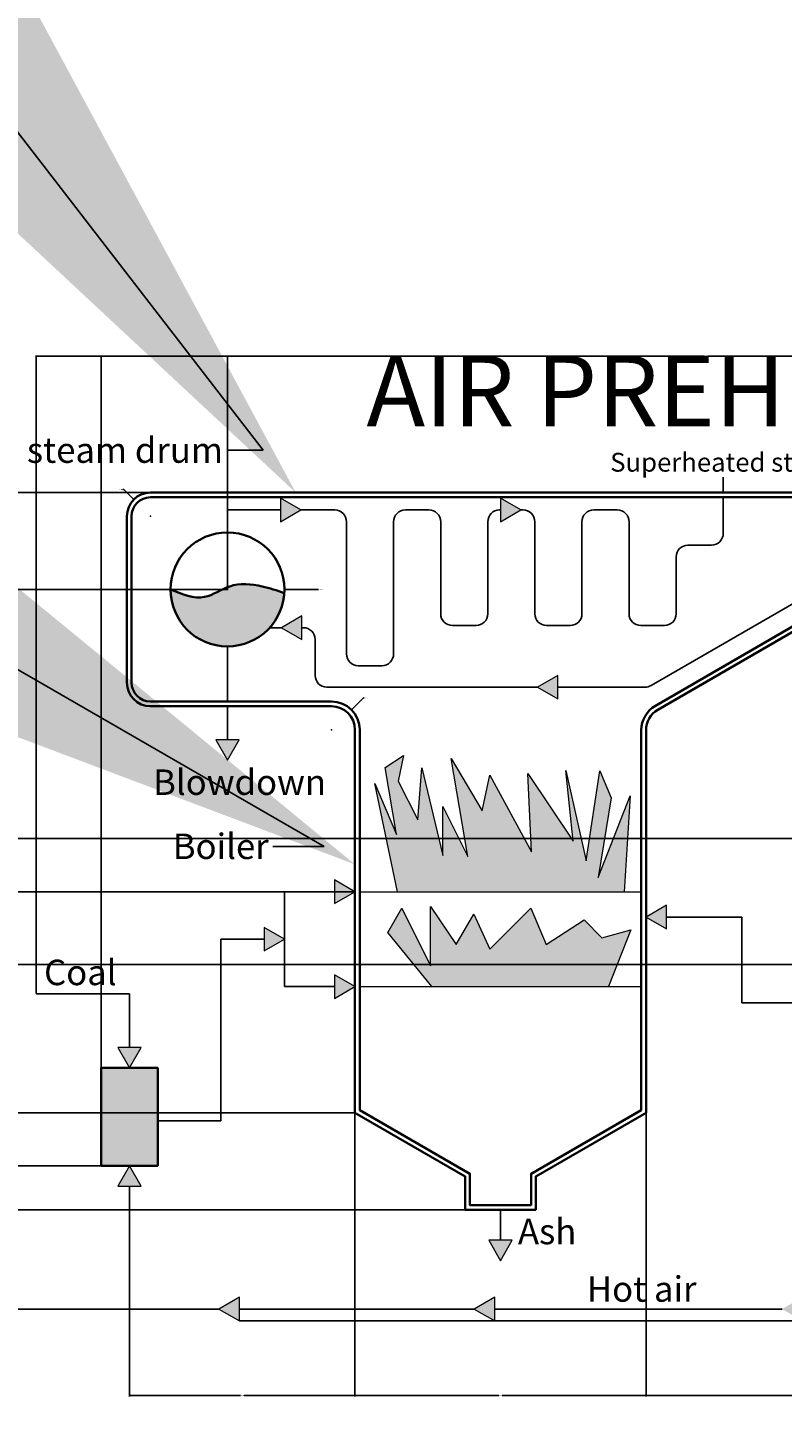
# Model space of a CAD drawing. Units: inches. Extents: x -9413 to 9703, y -9719 to 9096.
# Tile 1 of 1: x -0.3 to 159.8, y -19.4 to 276.8. Entities that reach past the tile are written whole.
import ezdxf
from ezdxf import colors
from ezdxf.entities.mleader import LeaderData, LeaderLine
from ezdxf.math import Vec2, Vec3

# ---------------------------------------------------------------- set-up
doc = ezdxf.new("R2010")
doc.units = ezdxf.units.IN
doc.header["$MEASUREMENT"] = 0
for name, color, linetype, lineweight in [('M-ANNO-TEXT', 7, 'Continuous', 18), ('M-ANNO-TITL', 7, 'Continuous', 35), ('M-DIMS', 2, 'Continuous', 18), ('M-DUCT-AIR', 4, 'Continuous', 25), ('M-EQPM', 7, 'Continuous', 35), ('M-EQPM-FIRE', 30, 'Continuous', 18), ('M-EQPM-PATT', 252, 'Continuous', 13), ('M-FLOW-PATT', 252, 'Continuous', 13), ('M-FLOW-SYMB', 7, 'Continuous', 18), ('M-PIPE-BWTR', 151, 'Continuous', 25), ('M-PIPE-STEM', 1, 'Continuous', 25), ('M-PROC-SOLD', 32, 'Continuous', 25)]:
    doc.layers.add(name, color=color, linetype=linetype, lineweight=lineweight)
doc.styles.get("Standard").update_dxf_attribs({"font": 'arial.ttf'})
doc.dimstyles.get("Standard").update_dxf_attribs({"dimtxt": 0.18, "dimasz": 0.18, "dimexe": 0.18, "dimexo": 0.0625, "dimgap": 0.09, "dimtad": 0, "dimtih": 1, "dimtoh": 1, "dimdec": 4, "dimzin": 0, "dimdsep": 46, "dimtxsty": 'Standard', "dimcen": 0.09, "dimadec": 0, "dimazin": 0, "dimtfac": 1, "dimtdec": 4, "dimtofl": 0, "dimtmove": 0, "dimatfit": 3, "dimfxl": 1, "dimtolj": 1, "dimtzin": 0, "dimarcsym": 0})

# ---------------------------------------------------------------- blocks, each defined once
blk = doc.blocks.new('FLOW-ARROW')
blk.add_lwpolyline([(0.000248294399313, -0.0003913674265164), (5.000248294399312, -0.0003913674265164), (2.500248294399312, 4.32973565149561)], close=True)
blk = doc.blocks.new('*D2')
at = {"layer": 'Defpoints', "color": 0, "transparency": 16777216}
for p in [(285.887484, 207.124736), (285.887484, 98.66208700000001), (1.37911, 71.85931899999999)]:
    blk.add_point(p, dxfattribs=at)
at = {"layer": 'M-DIMS', "color": 0, "lineweight": -2, "transparency": 16777216}
for p, q in [((1.37911, 71.921819), (1.379110000000008, 207.304736)), ((1.559110000000008, 207.124736), (143.2373829481582, 207.124736)), ((285.707484, 207.124736), (144.0292110518417, 207.124736)), ((285.887484, 98.72458700000001), (285.887484, 207.304736))]:
    blk.add_line(p, q, dxfattribs=at)
at = {"layer": 'M-DIMS', "color": 0, "transparency": 16777216}
for points in [[(1.559110000000008, 207.154736), (1.559110000000008, 207.094736), (1.379110000000008, 207.124736)], [(285.707484, 207.154736), (285.707484, 207.094736), (285.887484, 207.124736)]]:
    blk.add_solid(points, dxfattribs=at)
at = {"layer": 'M-DIMS', "color": 0, "transparency": 16777216, "insert": (143.633297, 207.124736), "char_height": 0.18, "attachment_point": 5}
blk.add_mtext('\\A1;284.5', dxfattribs=at)
blk = doc.blocks.new('*D3')
at = {"layer": 'Defpoints', "color": 0, "transparency": 16777216}
for p in [(234.2342480000001, 191.274736), (44.55608500000002, 2.461023), (301.7374840000002, 2.461023000000042)]:
    blk.add_point(p, dxfattribs=at)
at = {"layer": 'M-DIMS', "color": 0, "lineweight": -2, "transparency": 16777216}
for p, q in [((234.2967480000001, 191.274736), (301.9174840000002, 191.274736)), ((301.7374840000002, 191.094736), (301.7374840000002, 97.04978263778997)), ((301.7374840000002, 2.641023000000042), (301.7374840000002, 96.68597636221016)), ((44.61858500000001, 2.461023), (301.9174840000002, 2.461023000000042))]:
    blk.add_line(p, q, dxfattribs=at)
at = {"layer": 'M-DIMS', "color": 0, "transparency": 16777216}
for points in [[(301.7074840000002, 191.094736), (301.7674840000001, 191.094736), (301.7374840000002, 191.274736)], [(301.7074840000002, 2.641023000000042), (301.7674840000002, 2.641023000000042), (301.7374840000002, 2.461023000000042)]]:
    blk.add_solid(points, dxfattribs=at)
at = {"layer": 'M-DIMS', "color": 0, "transparency": 16777216, "insert": (301.7374840000002, 96.86787949999994), "char_height": 0.18, "attachment_point": 5}
blk.add_mtext('\\A1;188.8', dxfattribs=at)
blk = doc.blocks.new('*D4')
at = {"layer": 'Defpoints', "color": 0, "transparency": 16777216}
for p in [(69.11352, 46.59639499999999), (21.227159, 4.961022999999999), (69.11352, -13.388977)]:
    blk.add_point(p, dxfattribs=at)
at = {"layer": 'M-DIMS', "color": 0, "lineweight": -2, "transparency": 16777216}
for p, q in [((69.11352, 46.533895), (69.11352, -13.56897699999999)), ((21.227159, 4.898522999999999), (21.227159, -13.568977)), ((21.407159, -13.388977), (44.77282926807639, -13.388977)), ((68.93351999999999, -13.388977), (45.56784973192359, -13.388977))]:
    blk.add_line(p, q, dxfattribs=at)
at = {"layer": 'M-DIMS', "color": 0, "transparency": 16777216}
for points in [[(21.407159, -13.358977), (21.407159, -13.418977), (21.227159, -13.388977)], [(68.93351999999999, -13.358977), (68.93351999999999, -13.418977), (69.11352, -13.388977)]]:
    blk.add_solid(points, dxfattribs=at)
at = {"layer": 'M-DIMS', "color": 0, "transparency": 16777216, "insert": (45.1703395, -13.388977), "char_height": 0.18, "attachment_point": 5}
blk.add_mtext('\\A1;47.89', dxfattribs=at)
blk = doc.blocks.new('*D5')
at = {"layer": 'Defpoints', "color": 0, "transparency": 16777216}
for p in [(69.11352, 46.59639499999999), (130.910134, 46.59639499999999), (130.910134, -13.388977)]:
    blk.add_point(p, dxfattribs=at)
at = {"layer": 'M-DIMS', "color": 0, "lineweight": -2, "transparency": 16777216}
for p, q in [((69.11352, 46.533895), (69.11352, -13.56897699999999)), ((130.910134, 46.533895), (130.910134, -13.56897699999999)), ((69.29352, -13.388977), (99.68737270259209, -13.388977)), ((130.730134, -13.388977), (100.3362812974079, -13.388977))]:
    blk.add_line(p, q, dxfattribs=at)
at = {"layer": 'M-DIMS', "color": 0, "transparency": 16777216}
for points in [[(69.29352, -13.358977), (69.29352, -13.418977), (69.11352, -13.388977)], [(130.730134, -13.358977), (130.730134, -13.418977), (130.910134, -13.388977)]]:
    blk.add_solid(points, dxfattribs=at)
at = {"layer": 'M-DIMS', "color": 0, "transparency": 16777216, "insert": (100.011827, -13.388977), "char_height": 0.18, "attachment_point": 5}
blk.add_mtext('\\A1;61.8', dxfattribs=at)
blk = doc.blocks.new('*D6')
at = {"layer": 'Defpoints', "color": 0, "transparency": 16777216}
for p in [(221.144491, 80.86084099999998), (130.910134, 46.59639499999999), (221.144491, -13.388977)]:
    blk.add_point(p, dxfattribs=at)
at = {"layer": 'M-DIMS', "color": 0, "lineweight": -2, "transparency": 16777216}
for p, q in [((221.144491, 80.798341), (221.144491, -13.568977)), ((130.910134, 46.533895), (130.910134, -13.56897699999999)), ((131.090134, -13.388977), (175.6336085436562, -13.388977)), ((220.964491, -13.388977), (176.4210164563437, -13.388977))]:
    blk.add_line(p, q, dxfattribs=at)
at = {"layer": 'M-DIMS', "color": 0, "transparency": 16777216}
for points in [[(131.090134, -13.358977), (131.090134, -13.418977), (130.910134, -13.388977)], [(220.964491, -13.358977), (220.964491, -13.418977), (221.144491, -13.388977)]]:
    blk.add_solid(points, dxfattribs=at)
at = {"layer": 'M-DIMS', "color": 0, "transparency": 16777216, "insert": (176.0273125, -13.388977), "char_height": 0.18, "attachment_point": 5}
blk.add_mtext('\\A1;90.23', dxfattribs=at)
blk = doc.blocks.new('*D7')
at = {"layer": 'Defpoints', "color": 0, "transparency": 16777216}
for p in [(-14.47089000000002, 35.36125100000002), (15.22950700000001, 35.36125100000002), (21.22715900000001, 4.961023000000001)]:
    blk.add_point(p, dxfattribs=at)
at = {"layer": 'M-DIMS', "color": 0, "lineweight": -2, "transparency": 16777216}
for p, q in [((15.16700700000001, 35.36125100000002), (-14.65089000000001, 35.36125100000002)), ((-14.47089000000002, 35.18125100000002), (-14.47089000000001, 20.34310152933151)), ((-14.47089000000001, 5.141022999999995), (-14.47089000000001, 19.97917247066849)), ((21.16465900000001, 4.961023000000001), (-14.65089000000001, 4.961022999999995))]:
    blk.add_line(p, q, dxfattribs=at)
at = {"layer": 'M-DIMS', "color": 0, "transparency": 16777216}
for points in [[(-14.50089000000001, 35.18125100000002), (-14.44089000000001, 35.18125100000002), (-14.47089000000002, 35.36125100000002)], [(-14.50089000000001, 5.141022999999995), (-14.44089000000001, 5.141022999999995), (-14.47089000000001, 4.961022999999995)]]:
    blk.add_solid(points, dxfattribs=at)
at = {"layer": 'M-DIMS', "color": 0, "transparency": 16777216, "insert": (-14.47089, 20.161137), "char_height": 0.18, "attachment_point": 5}
blk.add_mtext('\\A1;30.4', dxfattribs=at)
blk = doc.blocks.new('*D8')
at = {"layer": 'Defpoints', "color": 0, "transparency": 16777216}
for p in [(-14.47089000000002, 93.50315200000001), (69.11352000000002, 93.50315200000001), (69.11352000000002, 46.59639500000001)]:
    blk.add_point(p, dxfattribs=at)
at = {"layer": 'M-DIMS', "color": 0, "lineweight": -2, "transparency": 16777216}
for p, q in [((69.05102000000002, 93.50315200000001), (-14.65089000000003, 93.50315200000001)), ((-14.47089000000002, 93.32315200000001), (-14.47089000000001, 70.23167663778992)), ((-14.47089000000001, 46.776395), (-14.47089000000001, 69.86787036221011)), ((69.05102000000002, 46.59639500000001), (-14.65089000000002, 46.596395))]:
    blk.add_line(p, q, dxfattribs=at)
at = {"layer": 'M-DIMS', "color": 0, "transparency": 16777216}
for points in [[(-14.50089000000002, 93.32315200000001), (-14.44089000000002, 93.32315200000001), (-14.47089000000002, 93.50315200000001)], [(-14.50089000000001, 46.776395), (-14.44089000000001, 46.776395), (-14.47089000000001, 46.596395)]]:
    blk.add_solid(points, dxfattribs=at)
at = {"layer": 'M-DIMS', "color": 0, "transparency": 16777216, "insert": (-14.47088999999999, 70.0497735), "char_height": 0.18, "attachment_point": 5}
blk.add_mtext('\\A1;46.91', dxfattribs=at)
blk = doc.blocks.new('*D9')
at = {"layer": 'Defpoints', "color": 0, "transparency": 16777216}
for p in [(-14.47089000000002, 178.191776), (25.67423200000002, 178.191776), (42.03736800000001, 157.648001)]:
    blk.add_point(p, dxfattribs=at)
at = {"layer": 'M-DIMS', "color": 0, "lineweight": -2, "transparency": 16777216}
for p, q in [((25.61173200000002, 178.191776), (-14.65089000000002, 178.191776)), ((-14.47089000000002, 178.011776), (-14.47089000000001, 168.1017916377899)), ((-14.47089000000001, 157.828001), (-14.47089000000001, 167.7379853622101)), ((41.97486800000001, 157.648001), (-14.65089000000001, 157.648001))]:
    blk.add_line(p, q, dxfattribs=at)
at = {"layer": 'M-DIMS', "color": 0, "transparency": 16777216}
for points in [[(-14.50089000000001, 178.011776), (-14.44089000000001, 178.011776), (-14.47089000000002, 178.191776)], [(-14.50089000000001, 157.828001), (-14.44089000000001, 157.828001), (-14.47089000000001, 157.648001)]]:
    blk.add_solid(points, dxfattribs=at)
at = {"layer": 'M-DIMS', "color": 0, "transparency": 16777216, "insert": (-14.47088999999996, 167.9198885), "char_height": 0.18, "attachment_point": 5}
blk.add_mtext('\\A1;20.544', dxfattribs=at)
blk = doc.blocks.new('*D10')
at = {"layer": 'Defpoints', "color": 0, "transparency": 16777216}
for p in [(42.037368, 207.124736), (42.037368, 157.648001), (15.229507, 56.137726)]:
    blk.add_point(p, dxfattribs=at)
at = {"layer": 'M-DIMS', "color": 0, "lineweight": -2, "transparency": 16777216}
for p, q in [((15.229507, 56.200226), (15.22950700000001, 207.304736)), ((15.40950700000001, 207.124736), (28.25557256139155, 207.124736)), ((41.85736799999999, 207.124736), (29.01130243860846, 207.124736)), ((42.037368, 157.710501), (42.037368, 207.304736))]:
    blk.add_line(p, q, dxfattribs=at)
at = {"layer": 'M-DIMS', "color": 0, "transparency": 16777216}
for points in [[(15.40950700000001, 207.154736), (15.40950700000001, 207.094736), (15.22950700000001, 207.124736)], [(41.85736799999999, 207.154736), (41.85736799999999, 207.094736), (42.037368, 207.124736)]]:
    blk.add_solid(points, dxfattribs=at)
at = {"layer": 'M-DIMS', "color": 0, "transparency": 16777216, "insert": (28.63343750000001, 207.124736), "char_height": 0.18, "attachment_point": 5}
blk.add_mtext('\\A1;26.81', dxfattribs=at)
blk = doc.blocks.new('*D13')
at = {"layer": 'Defpoints', "color": 0, "transparency": 16777216}
for p in [(-14.47089000000002, 104.790816), (234.0943920000001, 104.790816), (234.0943920000001, 78.04556900000003)]:
    blk.add_point(p, dxfattribs=at)
at = {"layer": 'M-DIMS', "color": 0, "lineweight": -2, "transparency": 16777216}
for p, q in [((234.0318920000001, 104.790816), (-14.65089000000003, 104.790816)), ((-14.47089000000002, 104.610816), (-14.47089000000001, 91.6000956377899)), ((-14.47089000000001, 78.225569), (-14.47089000000001, 91.23628936221009)), ((234.0318920000001, 78.04556900000003), (-14.65089000000002, 78.04556899999999))]:
    blk.add_line(p, q, dxfattribs=at)
at = {"layer": 'M-DIMS', "color": 0, "transparency": 16777216}
for points in [[(-14.50089000000002, 104.610816), (-14.44089000000002, 104.610816), (-14.47089000000002, 104.790816)], [(-14.50089000000001, 78.225569), (-14.44089000000001, 78.225569), (-14.47089000000001, 78.04556899999999)]]:
    blk.add_solid(points, dxfattribs=at)
at = {"layer": 'M-DIMS', "color": 0, "transparency": 16777216, "insert": (-14.47088999999999, 91.41819249999998), "char_height": 0.18, "attachment_point": 5}
blk.add_mtext('\\A1;26.745', dxfattribs=at)
blk = doc.blocks.new('*D17')
at = {"layer": 'Defpoints', "color": 0, "transparency": 16777216}
for p in [(92.51182700000003, 26.01294900000001), (-14.47089000000001, 4.961022999999995), (21.22715900000001, 4.961023000000001)]:
    blk.add_point(p, dxfattribs=at)
at = {"layer": 'M-DIMS', "color": 0, "lineweight": -2, "transparency": 16777216}
for p, q in [((92.44932700000003, 26.01294900000001), (-14.65089000000002, 26.012949)), ((-14.47089000000002, 25.832949), (-14.47089000000001, 15.6688891377899)), ((-14.47089000000001, 5.141022999999995), (-14.47089000000001, 15.30508286221009)), ((21.16465900000001, 4.961023000000001), (-14.65089000000001, 4.961022999999995))]:
    blk.add_line(p, q, dxfattribs=at)
at = {"layer": 'M-DIMS', "color": 0, "transparency": 16777216}
for points in [[(-14.50089000000001, 25.832949), (-14.44089000000001, 25.832949), (-14.47089000000002, 26.012949)], [(-14.50089000000001, 5.141022999999995), (-14.44089000000001, 5.141022999999995), (-14.47089000000001, 4.961022999999995)]]:
    blk.add_solid(points, dxfattribs=at)
at = {"layer": 'M-DIMS', "color": 0, "transparency": 16777216, "insert": (-14.47089, 15.48698599999999), "char_height": 0.18, "attachment_point": 5}
blk.add_mtext('\\A1;21.05', dxfattribs=at)
blk = doc.blocks.new('*D18')
at = {"layer": 'Defpoints', "color": 0, "transparency": 16777216}
for p in [(29.951966, 157.648002), (54.12277, 157.648)]:
    blk.add_point(p, dxfattribs=at)
at = {"layer": 'M-DIMS', "color": 0, "lineweight": -2, "transparency": 16777216}
for p, q in [((41.947368, 157.648001), (42.127368, 157.648001)), ((42.037368, 157.558001), (42.037368, 157.738001)), ((61.37401119999997, 157.6479994), (54.30277, 157.647999985106))]:
    blk.add_line(p, q, dxfattribs=at)
at = {"layer": 'M-DIMS', "color": 0, "transparency": 16777216}
blk.add_solid([(54.30277000248233, 157.677999985106), (54.30276999751766, 157.617999985106), (54.12277, 157.648)], dxfattribs=at)
at = {"layer": 'M-DIMS', "color": 0, "transparency": 16777216, "insert": (61.86563466521143, 157.6479994), "char_height": 0.18, "attachment_point": 5}
blk.add_mtext('\\A1;∅24.17', dxfattribs=at)
blk = doc.blocks.new('*D19')
at = {"layer": 'Defpoints', "color": 0, "transparency": 16777216}
for p in [(68.35624600000001, 132.114246), (64.11352, 127.87169)]:
    blk.add_point(p, dxfattribs=at)
at = {"layer": 'M-DIMS', "color": 0, "lineweight": -2, "transparency": 16777216}
for p, q in [((70.9018814117569, 134.6597794117645), (68.48352777058787, 132.2415226705882)), ((71.08188141175692, 134.6597794117645), (70.9018814117569, 134.6597794117645)), ((64.02352000000002, 127.87169), (64.20352000000004, 127.87169)), ((64.11352000000004, 127.78169), (64.11352000000002, 127.96169))]:
    blk.add_line(p, q, dxfattribs=at)
at = {"layer": 'M-DIMS', "color": 0, "transparency": 16777216}
blk.add_solid([(68.4623149921565, 132.2627362990195), (68.50474054901923, 132.2203090421569), (68.35624600000001, 132.114246)], dxfattribs=at)
at = {"layer": 'M-DIMS', "color": 0, "transparency": 16777216, "insert": (71.51186776919214, 134.6597794117645), "char_height": 0.18, "attachment_point": 5}
blk.add_mtext('\\A1;2X R6', dxfattribs=at)
blk = doc.blocks.new('*D20')
at = {"layer": 'Defpoints', "color": 0, "transparency": 16777216}
for p in [(22.138694, 176.727306), (25.67423199999999, 173.191776)]:
    blk.add_point(p, dxfattribs=at)
at = {"layer": 'M-DIMS', "color": 0, "lineweight": -2, "transparency": 16777216}
for p, q in [((19.83737125644178, 178.8486239435583), (20.01737125644179, 178.8486239435583)), ((20.01737125644179, 178.8486239435583), (22.0114146353865, 176.8545850766135)), ((25.584232, 173.191776), (25.76423199999999, 173.191776)), ((25.674232, 173.101776), (25.67423199999999, 173.281776))]:
    blk.add_line(p, q, dxfattribs=at)
at = {"layer": 'M-DIMS', "color": 0, "transparency": 16777216}
blk.add_solid([(22.03262781482209, 176.8757983040491), (21.99020145595092, 176.8333718491779), (22.138694, 176.727306)], dxfattribs=at)
at = {"layer": 'M-DIMS', "color": 0, "transparency": 16777216, "insert": (19.40891968754683, 178.8486239435583), "char_height": 0.18, "attachment_point": 5}
blk.add_mtext('\\A1;7X R5', dxfattribs=at)

msp = doc.modelspace()

# ---------------------------------------------------------------- hatches: boundary and pattern name
at = {"layer": 'M-EQPM-PATT'}
h = msp.add_hatch(color=256, dxfattribs=at)
h.set_gradient(color1=(173, 221, 247), color2=(39, 118, 187), tint=1, name='CYLINDER')
edge = h.paths.add_edge_path()
edge.add_spline(control_points=[(54.09820106687558, 156.8777785228646), (52.55234687665725, 157.4038723263632), (48.84690877622666, 158.6649278878898), (42.66912031574928, 159.2097831474938), (36.81636607490111, 154.7692159506864), (32.42236659770719, 156.6119671913352), (29.9519659208658, 157.6480014320714)], knot_values=[0, 0, 0, 0, 4.924664268089502, 11.80450182577105, 17.57703903378495, 24.99047671276265, 24.99047671276265, 24.99047671276265, 24.99047671276265], degree=3, periodic=0)
edge.add_arc((42.03736787953743, 157.6480014320714), 12.08540195867163, 180.0000000000001, 356.34596753837)
h = msp.add_hatch(color=256, dxfattribs=at)
h.set_gradient(color1=(248, 153, 30), color2=(237, 31, 36), tint=1)
h.paths.add_polyline_path([(87.75589157594366, 101.2079377323113), (83.33266595518216, 119.7615608844223), (82.44795815245014, 108.7809173188158), (78.27764050074619, 116.9847978998165), (79.43704609243808, 122.4462941906285), (75.49721980444154, 119.8877410833244), (77.8984352435218, 105.6254996505174), (73.34891233453526, 116.4799630172362), (78.15134321257936, 93.50315249510626), (126.3010091031319, 93.50315249510626), (127.5646087703644, 113.8294943185043), (120.7401677105226, 96.53801541630102), (123.5205884068272, 113.4508396348262), (121.1193729678052, 119.1304317159826), (118.2126549833337, 100.0720877682631), (113.916040043463, 119.2567260018565), (115.4325476798112, 104.2371752017076), (105.8276859236648, 118.6255968334023), (106.5860964381718, 101.9652470996531), (97.73964519659056, 118.2469421497241), (96.09684027213369, 110.6740766502059), (89.52530718140768, 121.7810145017008), (93.0638249994954, 100.955577334507), (87.75589157594366, 111.5575662164498)])
h.paths.add_polyline_path([(97.74371930269989, 81.31367848864618), (94.3518728191552, 88.73363375012146), (90.62750956969101, 82.28284737620714), (85.1284065536456, 90.35906462757129), (85.1284065536456, 77.76009726325145), (79.05941859470452, 90.04219422748807), (76.07166876032714, 84.86725971404093), (85.45214128983207, 73.3852454047991), (122.9248287422815, 73.3852454047991), (127.6846966755432, 85.39453008026015), (121.5263470998272, 83.74440528473849), (117.7608440325205, 87.50990835204513), (109.7118759721052, 82.28284737620714), (106.4711964161688, 90.04115560211511)])
h = msp.add_hatch(color=256, dxfattribs=at)
h.set_gradient(color1=(247, 171, 174), color2=(241, 235, 31), tint=1, name='CYLINDER')
h.paths.add_polyline_path([(234.0943920106286, 104.7908162978576), (234.0943920106286, 96.56150977514116), (240.6285668506998, 96.56150977514116), (240.6285668506998, 86.27487600315693), (234.0943920106286, 86.27487600315693), (234.0943920106286, 78.04556948044049), (251.1627416907711, 78.04556948044049), (251.1627416907711, 86.27487600315693), (244.6285668506998, 86.27487600315693), (244.6285668506998, 96.56150977514116), (251.1627416907711, 96.56150977514116), (251.1627416907711, 104.7908162978576)])
h.paths.add_polyline_path([(27.22481035966126, 56.13772641082374), (15.22950676080154, 56.13772641082374), (15.22950676080154, 35.36125112538483), (27.22481035966124, 35.36125112538483)])
at = {"layer": 'M-FLOW-PATT'}
h = msp.add_hatch(color=256, dxfattribs=at)
h.set_gradient(color1=(0, 0, 255), color2=(237, 31, 36), tint=1, name='CYLINDER')
h.paths.add_polyline_path([(57.60719326604156, 174.5154936822842), (53.27706624711947, 177.0154936822843), (53.27706624711947, 172.0154936822843)])
h.paths.add_polyline_path([(104.3199532850412, 174.5154936822842), (99.98982626611915, 177.0154936822843), (99.98982626611915, 172.0154936822843)])
h.paths.add_polyline_path([(53.52042794230806, 149.5365959733167), (57.85055496123027, 147.0365959733168), (57.85055496123027, 152.0365959733167)])
h.paths.add_polyline_path([(39.53736787953737, 125.7512816544064), (42.03736787953743, 121.4211546354843), (44.53736787953743, 125.7512816544064)])
h.paths.add_polyline_path([(112.1909801989792, 134.4074487017934), (112.1909801989792, 139.4074487017932), (107.860853180057, 136.9074487017932)])
h.paths.add_polyline_path([(177.2741254076526, 153.9161106668102), (177.2741254076526, 158.9161106668101), (172.9439983887304, 156.4161106668101)])
h.paths.add_polyline_path([(49.82189913347245, 85.9441989499526), (49.82189913347245, 80.94419894995266), (54.15202615239467, 83.44419894995269)])
h.paths.add_polyline_path([(69.11352005531556, 93.50315249510626), (64.78339303639335, 96.0031524951062), (64.78339303639335, 91.00315249510626)])
h.paths.add_polyline_path([(69.11352005531553, 73.38524540479911), (64.78339303639335, 75.885245404799), (64.78339303639335, 70.88524540479908)])
h.paths.add_polyline_path([(18.72715856023135, 60.46785342974584), (21.22715856023142, 56.13772641082373), (23.72715856023141, 60.46785342974583)])
h.paths.add_polyline_path([(21.22715856023142, 35.36125112538483), (18.72715856023142, 31.0311241064627), (23.72715856023143, 31.03112410646267)])
h.paths.add_polyline_path([(44.55608540223805, 7.461022688866137), (40.22595838331583, 4.961022688866137), (44.55608540223805, 2.461022688866222)])
h.paths.add_polyline_path([(98.78154953768238, 2.461022688866194), (98.78154953768238, 7.461022688866137), (94.45142251876013, 4.961022688866108)])
h.paths.add_polyline_path([(97.51182696160306, 19.53928695608056), (100.0118269616031, 15.20915993715846), (102.5118269616031, 19.53928695608053)])
h.paths.add_polyline_path([(164.1352451136813, 2.461022688866222), (164.1352451136813, 7.461022688866108), (159.8051180947591, 4.961022688866165)])
h.paths.add_polyline_path([(209.3801796746353, 46.61055823726996), (211.8801796746354, 42.28043121834784), (214.3801796746354, 46.61055823726991)])
h.paths.add_polyline_path([(183.686965899029, 72.398812257232), (179.3568388801068, 69.89881225723198), (183.686965899029, 67.3988122572321)])
h.paths.add_polyline_path([(130.9101338678906, 88.12957450655973), (135.2402608868128, 85.6295745065598), (135.2402608868128, 90.62957450655973)])
h.paths.add_polyline_path([(235.6787428099642, 114.793018678795), (231.348615791042, 112.293018678795), (235.6787428099642, 109.7930186787951)])
h.paths.add_polyline_path([(234.0943920106286, 97.87236613613993), (229.7642649917063, 100.3723661361398), (229.7642649917063, 95.37236613613992)])
h.paths.add_polyline_path([(235.6787428099642, 139.7381753554388), (231.348615791042, 137.2381753554388), (235.6787428099642, 134.7381753554389)])
h.paths.add_polyline_path([(234.2342482943993, 191.2747356514956), (231.7342482943993, 186.9446086325734), (236.7342482943993, 186.9446086325734)])
h.paths.add_polyline_path([(281.5573566069943, 96.1620867934123), (285.8874836259165, 98.6620867934123), (281.5573566069943, 101.1620867934122)])
h.paths.add_polyline_path([(282.8693181059843, 72.82025870979582), (278.539191087062, 70.32025870979582), (282.8693181059843, 67.8202587097959)])
h.paths.add_polyline_path([(255.4928687096933, 79.6602227417988), (255.4928687096933, 84.66022274179872), (251.1627416907711, 82.16022274179872)])

# ---------------------------------------------------------------- linework, layer by layer
at = {"layer": 'M-DUCT-AIR'}
for p, q in [((151.2395643983297, 88.12957450655972), (135.2402608868128, 88.12957450655972)), ((151.2395643983297, 69.898812257232), (151.2395643983297, 88.12957450655972)), ((179.3568388801068, 69.898812257232), (151.2395643983297, 69.898812257232)), ((21.2271585602314, 31.0311241064627), (21.22715856023139, 4.961022688866137)), ((21.22715856023139, 4.961022688866137), (40.22595838331584, 4.961022688866137)), ((44.55608540223805, 4.961022688866137), (94.45142251876017, 4.961022688866137)), ((98.78154953768238, 4.961022688866137), (159.8051180947591, 4.961022688866137))]:
    msp.add_line(p, q, dxfattribs=at)
at = {"layer": 'M-EQPM'}
for points in [[(71.38513555915277, 178.1917761520126), (25.67423247811051, 178.1917761520126, 0.4142135623730951), (20.67423247811051, 173.1917761520126), (20.67423247811051, 137.8716904891279, 0.4142135623730951), (25.67423247811051, 132.8716904891279), (64.11352005531556, 132.8716904891279, -0.4142135623730951), (69.11352005531556, 127.8716904891279), (69.11352005531555, 46.5963952605125), (92.51182696160309, 33.0873764695859), (92.51182696160309, 26.01294921083763), (107.5118269616031, 26.01294921083763), (107.5118269616031, 33.0873764695859), (130.9101338678906, 46.5963952605125), (130.9101338678906, 127.7737662120324, -0.267949192431123), (133.4101338678906, 132.1038932309546), (165.458308006557, 150.6069151969495)], [(71.38513555915277, 177.1917761520126), (25.67423247811051, 177.1917761520126, 0.4142135623730951), (21.67423247811052, 173.1917761520126), (21.67423247811051, 137.8716904891279, 0.4142135623730951), (25.67423247811051, 133.8716904891279), (64.11352005531556, 133.8716904891279, -0.4142135623730951), (70.11352005531556, 127.8716904891279), (70.11352005531555, 47.17374552970224), (93.51182696160309, 33.66472673877554), (93.51182696160309, 27.01294921083752), (106.5118269616031, 27.01294921083763), (106.5118269616031, 33.66472673877554), (129.9101338678906, 47.17374552970209), (129.9101338678906, 127.7737662120324, -0.2679491924311227), (132.9101338678906, 132.969918634739), (165.1903588141258, 151.6069151969495)]]:
    msp.add_lwpolyline(points, format="xyb", dxfattribs=at)
for points in [[(216.1444910066821, 178.1917761520126), (56.5363078524973, 178.1917761520126)], [(216.1444910066821, 177.1917761520126), (71.38513555915277, 177.1917761520126)]]:
    msp.add_lwpolyline(points, dxfattribs=at)
msp.add_lwpolyline([(15.22950676080152, 56.13772641082374), (27.22481035966128, 56.13772641082374), (27.22481035966128, 35.36125112538483), (15.22950676080152, 35.36125112538483)], close=True, dxfattribs=at)
msp.add_circle((42.03736787953743, 157.6480014320714), 12.08540195867163, dxfattribs=at)
msp.add_open_spline([(29.9519659208658, 157.6480014320714), (32.42236659770719, 156.6119671913353), (36.8163660749011, 154.7692159506864), (42.66912031574928, 159.2097831474938), (48.84690877622666, 158.6649278878897), (52.55234687665726, 157.4038723263632), (54.09820106687558, 156.8777785228646)], degree=3, knots=[0, 0, 0, 0, 7.413437678977692, 13.1859748869916, 20.06581244467315, 24.99047671276265, 24.99047671276265, 24.99047671276265, 24.99047671276265], dxfattribs=at)
at = {"layer": 'M-EQPM-FIRE'}
for p, q in [((75.49721980444154, 119.8877410833244), (79.43704609243808, 122.4462941906285)), ((79.43704609243808, 122.4462941906285), (78.27764050074619, 116.9847978998165)), ((93.0638249994954, 100.955577334507), (89.52530718140768, 121.7810145017008)), ((89.52530718140768, 121.7810145017008), (96.09684027213369, 110.6740766502059)), ((77.8984352435218, 105.6254996505174), (75.49721980444154, 119.8877410833244)), ((82.44795815245014, 108.7809173188158), (83.33266595518216, 119.7615608844223)), ((83.33266595518216, 119.7615608844223), (87.75589157594366, 101.2079377323113)), ((106.5860964381718, 101.9652470996531), (105.8276859236648, 118.6255968334023)), ((105.8276859236648, 118.6255968334023), (115.4325476798112, 104.2371752017076)), ((115.4325476798112, 104.2371752017076), (113.916040043463, 119.2567260018565)), ((113.916040043463, 119.2567260018565), (118.2126549833337, 100.0720877682631)), ((118.2126549833337, 100.0720877682631), (121.1193729678052, 119.1304317159826)), ((121.1193729678052, 119.1304317159826), (123.5205884068273, 113.4508396348262)), ((78.15134321257936, 93.50315249510629), (73.34891233453526, 116.4799630172362)), ((73.34891233453526, 116.4799630172362), (77.8984352435218, 105.6254996505174)), ((78.27764050074619, 116.9847978998165), (82.44795815245014, 108.7809173188158)), ((96.09684027213369, 110.6740766502059), (97.73964519659056, 118.2469421497241)), ((97.73964519659056, 118.2469421497241), (106.5860964381718, 101.9652470996531)), ((120.7401677105226, 96.538015416301), (127.5646087703644, 113.8294943185043)), ((123.5205884068273, 113.4508396348262), (120.7401677105226, 96.538015416301)), ((127.5646087703644, 113.8294943185043), (126.3010091031319, 93.50315249510626)), ((87.75589157594366, 101.2079377323113), (87.75589157594366, 111.5575662164498)), ((87.75589157594366, 111.5575662164498), (93.0638249994954, 100.955577334507)), ((70.11352005531556, 93.50315249510626), (129.9101338678906, 93.50315249510626)), ((76.07166876032714, 84.86725971404093), (79.05941859470452, 90.04219422748807)), ((79.05941859470452, 90.04219422748807), (85.1284065536456, 77.76009726325145)), ((85.1284065536456, 77.76009726325145), (85.1284065536456, 90.35906462757129)), ((85.1284065536456, 90.35906462757129), (90.62750956969101, 82.28284737620714)), ((97.74371930269989, 81.31367848864618), (106.4711964161688, 90.04115560211511)), ((106.4711964161688, 90.04115560211511), (109.7118759721052, 82.28284737620714)), ((90.62750956969101, 82.28284737620714), (94.3518728191552, 88.73363375012146)), ((94.3518728191552, 88.73363375012146), (97.74371930269989, 81.31367848864618)), ((109.7118759721052, 82.28284737620714), (117.7608440325205, 87.50990835204513)), ((117.7608440325205, 87.50990835204513), (121.5263470998272, 83.74440528473849)), ((85.45214128983207, 73.3852454047991), (76.07166876032714, 84.86725971404093)), ((121.5263470998272, 83.74440528473849), (127.6846966755432, 85.39453008026015)), ((127.6846966755432, 85.39453008026015), (122.9248287422815, 73.3852454047991)), ((70.11352005531555, 73.3852454047991), (129.9101338678906, 73.3852454047991))]:
    msp.add_line(p, q, dxfattribs=at)
at = {"layer": 'M-PIPE-BWTR'}
for p, q in [((131.9759748067024, 137.2423851923322), (164.6057144799537, 156.0811741762712)), ((50.99627640604608, 149.5365959733167), (53.52042794230806, 149.5365959733167)), ((57.85055496123027, 149.5365959733167), (58.14568900529365, 149.5365959733167)), ((42.03736787953743, 145.5625994733997), (42.03736787953742, 133.8716904891279)), ((60.64568900529365, 147.0365959733167), (60.64568900529365, 139.4074487017933)), ((63.14568900529365, 136.9074487017933), (107.8608531800571, 136.9074487017933)), ((112.1909801989792, 136.9074487017933), (130.7259748067023, 136.9074487017933)), ((42.03736787953742, 132.8716904891279), (42.03736787953742, 125.7512816544064))]:
    msp.add_line(p, q, dxfattribs=at)
for centre, start, end in [((58.14568900529365, 147.0365959733167), 0, 90), ((63.14568900529365, 139.4074487017933), 180, 270), ((130.7259748067023, 139.4074487017933), 270, 300)]:
    msp.add_arc(centre, 2.5, start, end, dxfattribs=at)
at = {"layer": 'M-PIPE-STEM'}
for p, q in [((147.30818160586, 178.1917761520126), (147.30818160586, 181.458788950076)), ((99.80818160586, 174.5154936822842), (99.98982626611915, 174.5154936822842)), ((104.3199532850412, 174.5154936822842), (104.80818160586, 174.5154936822842)), ((89.80818160585999, 149.9883982653171), (94.80818160585999, 149.9883982653171)), ((109.80818160586, 149.9883982653171), (114.80818160586, 149.9883982653171)), ((129.80818160586, 149.9883982653171), (134.80818160586, 149.9883982653171))]:
    msp.add_line(p, q, dxfattribs=at)
for points in [[(147.30818160586, 177.1917761520126), (147.30818160586, 169.5494691851729, -0.4142135623730951), (144.80818160586, 167.0494691851729), (139.80818160586, 167.0494691851729, 0.4142135623730951), (137.30818160586, 164.5494691851729), (137.30818160586, 152.4883982653172)], [(57.60719326604156, 174.5154936822842), (64.80818160585999, 174.5154936822842, -0.4142135623730951), (67.30818160585999, 172.0154936822843), (67.30818160585999, 143.9616554963527, 0.4142135623730951), (69.80818160585999, 141.4616554963527), (74.80818160586, 141.4616554963527, 0.4142135623730951), (77.30818160586, 143.9616554963527), (77.30818160585999, 172.0154936822843, -0.4142135623730953), (79.80818160585999, 174.5154936822842), (84.80818160585999, 174.5154936822842, -0.4142135623730951), (87.30818160585999, 172.0154936822843), (87.30818160585999, 152.4883982653172)], [(97.30818160585999, 152.4883982653172), (97.30818160586, 172.0154936822843, -0.4142135623730948), (99.80818160586, 174.5154936822842)], [(104.80818160586, 174.5154936822842, -0.4142135623730951), (107.30818160586, 172.0154936822843), (107.30818160586, 152.4883982653172)], [(117.30818160586, 152.4883982653172), (117.30818160586, 172.0154936822843, -0.4142135623730951), (119.80818160586, 174.5154936822842), (124.80818160586, 174.5154936822842, -0.4142135623730951), (127.30818160586, 172.0154936822843), (127.30818160586, 152.4883982653172)]]:
    msp.add_lwpolyline(points, format="xyb", dxfattribs=at)
msp.add_lwpolyline([(42.03736787953743, 169.733403390743), (42.03736787953743, 174.5154936822842), (53.27706624711947, 174.5154936822842)], dxfattribs=at)
for centre, start, end in [((89.80818160585999, 152.4883982653172), 180, 270), ((94.80818160585999, 152.4883982653172), 270, 0), ((109.80818160586, 152.4883982653172), 180, 270), ((114.80818160586, 152.4883982653172), 270, 0), ((129.80818160586, 152.4883982653172), 180, 270), ((134.80818160586, 152.4883982653172), 270, 0)]:
    msp.add_arc(centre, 2.5, start, end, dxfattribs=at)
at = {"layer": 'M-PROC-SOLD'}
for p, q in [((64.78339303639335, 93.50315249510626), (54.15202615239467, 93.50315249510626)), ((54.15202615239467, 93.50315249510626), (54.15202615239466, 73.38524540479908)), ((49.82189913347245, 83.44419894995266), (40.6425727526332, 83.44419894995266)), ((40.6425727526332, 83.44419894995266), (40.64257275263319, 44.85937348128527)), ((21.2271585602314, 71.85931924224388), (1.379109573500485, 71.85931924224388)), ((21.2271585602314, 60.46785342974586), (21.2271585602314, 71.85931924224388)), ((54.15202615239466, 73.38524540479908), (64.78339303639335, 73.38524540479906)), ((40.64257275263319, 44.85937348128527), (27.22481035966128, 44.85937348128527)), ((100.0118269616031, 26.01294921083763), (100.0118269616031, 19.53928695608056))]:
    msp.add_line(p, q, dxfattribs=at)

# ---------------------------------------------------------------- block references
at = {"layer": 'M-FLOW-SYMB'}
for p, rotation in [((53.27745761454611, 177.0157419766835), 269.9999999999983), ((99.9902176335458, 177.0157419766836), 269.9999999999981), ((57.85096567420092, 152.0363811863827), 210.0000000000003), ((112.1913909119498, 139.4072339148593), 210.0000000000008), ((44.53761617393673, 125.7508902869798), 180), ((64.78298232342269, 91.00336728204029), 30.00000000000032), ((135.2406715997834, 90.62935971962575), 210.0000000000003), ((49.82148842050175, 80.94441373688657), 30.00000000000027), ((64.78298232342269, 70.88546019173307), 30.00000000000032), ((23.72740685463069, 60.46746206231927), 180), ((102.5120752560024, 19.53889558865398), 180), ((44.55649611520875, 7.460807901932184), 210.0000000000004), ((98.78196025065309, 7.460807901932184), 210.0000000000004)]:
    msp.add_blockref('FLOW-ARROW', p, dxfattribs=dict(at, rotation=rotation))
msp.add_blockref('FLOW-ARROW', (18.72691026583214, 31.0315154738893), dxfattribs=at)

# ---------------------------------------------------------------- texts
at = {"layer": 'M-ANNO-TEXT', "attachment_point": 1}
for s, width, heights, insert, char_height in [('Superheated steam', 70.22066543495748, [13.99584833657717], (123.307481320051, 186.6375065489846), 4), ('Blowdown', 34.70919302415428, [0], (26.23367270059553, 119.4505937692062), 5.4), ('Coal', 17.34622007799442, [0], (3.09005014468731, 79.08116987591995), 5.4), ('Ash', 8.310862989805173, [0], (103.7144784444826, 24.11514472781135), 5.4), ('Hot air', 27.52518381383822, [0], (118.345597348535, 11.91022110372515), 5.4)]:
    msp.add_mtext_dynamic_manual_height_columns(s, width=width, gutter_width=1, heights=heights, dxfattribs=dict(at, insert=insert, char_height=char_height))
at = {"layer": 'M-ANNO-TITL', "insert": (71.55599227099447, 207.2732170699019), "char_height": 15, "attachment_point": 1}
msp.add_mtext_dynamic_manual_height_columns('AIR PREHEATER', width=207.9937702218885, gutter_width=1, heights=[0], dxfattribs=at)

# ---------------------------------------------------------------- dimensions: what is measured, and where the dimension line sits
at = {"layer": 'M-DIMS'}
for base, p1, p2, override, picture, middle in [((285.887484, 207.124736), (1.37911, 71.85931899999999), (285.887484, 98.66208700000001), {"dimdec": 1, "dimlfac": 1, "dimrnd": 0, "dimzin": 0, "dimdsep": 46, "dimlunit": 2}, '*D2', (143.633297, 207.124736)), ((42.037368, 207.124736), (15.229507, 56.137726), (42.037368, 157.648001), {"dimdec": 2, "dimlfac": 1, "dimrnd": 0, "dimzin": 0, "dimdsep": 46, "dimlunit": 2}, '*D10', (28.63343750000001, 207.124736)), ((221.144491, -13.388977), (130.910134, 46.59639499999999), (221.144491, 80.86084099999998), {"dimdec": 2, "dimlfac": 1, "dimrnd": 0, "dimzin": 0, "dimdsep": 46, "dimlunit": 2}, '*D6', (176.0273125, -13.388977)), ((69.11352, -13.388977), (21.227159, 4.961022999999999), (69.11352, 46.59639499999999), {"dimdec": 2, "dimlfac": 1, "dimrnd": 0, "dimzin": 0, "dimdsep": 46, "dimlunit": 2}, '*D4', (45.1703395, -13.388977)), ((130.910134, -13.388977), (69.11352, 46.59639499999999), (130.910134, 46.59639499999999), {"dimdec": 1, "dimlfac": 1, "dimrnd": 0, "dimzin": 0, "dimdsep": 46, "dimlunit": 2}, '*D5', (100.011827, -13.388977))]:
    dim = msp.add_linear_dim(base=base, p1=p1, p2=p2, dimstyle='Standard', override=override, dxfattribs=at)
    dim.commit()
    dim.dimension.update_dxf_attribs({"geometry": picture, "text_midpoint": middle})
for base, p1, p2, override, picture, middle in [((301.7374840000002, 2.461023000000042), (234.234248, 191.274736), (44.556085, 2.461022999999999), {"dimdec": 1, "dimlfac": 1, "dimrnd": 0, "dimzin": 0, "dimdsep": 46, "dimlunit": 2}, '*D3', (301.7374840000002, 96.86787949999994)), ((-14.47089000000002, 178.191776), (42.037368, 157.648001), (25.674232, 178.191776), {"dimdec": 3, "dimlfac": 1, "dimrnd": 0, "dimzin": 0, "dimdsep": 46, "dimlunit": 2}, '*D9', (-14.47088999999996, 167.9198885)), ((-14.47089000000002, 104.790816), (234.094392, 78.045569), (234.094392, 104.790816), {"dimdec": 3, "dimlfac": 1, "dimrnd": 0, "dimzin": 0, "dimdsep": 46, "dimlunit": 2}, '*D13', (-14.47088999999999, 91.41819249999998)), ((-14.47089000000002, 93.50315200000001), (69.11352, 46.59639499999999), (69.11352, 93.503152), {"dimdec": 2, "dimlfac": 1, "dimrnd": 0, "dimzin": 0, "dimdsep": 46, "dimlunit": 2}, '*D8', (-14.47088999999999, 70.0497735)), ((-14.47089000000002, 35.36125100000002), (21.227159, 4.961022999999999), (15.229507, 35.361251), {"dimdec": 1, "dimlfac": 1, "dimrnd": 0, "dimzin": 0, "dimdsep": 46, "dimlunit": 2}, '*D7', (-14.47089, 20.161137)), ((-14.47089000000001, 4.961022999999995), (92.511827, 26.012949), (21.227159, 4.961022999999999), {"dimdec": 2, "dimlfac": 1, "dimrnd": 0, "dimzin": 0, "dimdsep": 46, "dimlunit": 2}, '*D17', (-14.47089, 15.48698599999999))]:
    dim = msp.add_linear_dim(base=base, p1=p1, p2=p2, angle=90, dimstyle='Standard', override=override, dxfattribs=at)
    dim.commit()
    dim.dimension.update_dxf_attribs({"geometry": picture, "text_midpoint": middle})
for center, mpoint, text, picture, middle in [((25.67423199999999, 173.191776), (22.138694, 176.727306), '7X <>', '*D20', (19.40891968754683, 178.8486239435583)), ((64.11352, 127.87169), (68.35624600000001, 132.114246), '2X <>', '*D19', (71.51186776919214, 134.6597794117645))]:
    dim = msp.add_radius_dim(center=center, mpoint=mpoint, text=text, dimstyle='Standard', override={"dimdec": 0, "dimlfac": 1, "dimrnd": 0, "dimzin": 0, "dimdsep": 46, "dimlunit": 2}, dxfattribs=at)
    dim.commit()
    dim.dimension.update_dxf_attribs({"geometry": picture, "text_midpoint": middle, "dimtype": 164})
dim = msp.add_diameter_dim_2p(p1=(29.951966, 157.648002), p2=(54.12277, 157.648), dimstyle='Standard', override={"dimdec": 2, "dimlfac": 1, "dimrnd": 0, "dimzin": 0, "dimdsep": 46, "dimlunit": 2}, dxfattribs=at)
dim.commit()
dim.dimension.update_dxf_attribs({"geometry": '*D18', "text_midpoint": (61.37401119999997, 157.6479994), "dimtype": 163})

# ---------------------------------------------------------------- leaders
at = {"layer": 'M-ANNO-TEXT'}
ml = msp.add_multileader_mtext('Standard', dxfattribs=at)
ml.set_content('steam drum', color=256)
ml.set_leader_properties()
ml.build(insert=Vec2(0, 0))
ml.multileader.update_dxf_attribs({"dogleg_length": 0.36, "arrow_head_size": 10000, "scale": 10})
ctx = ml.context
ctx.base_point, ctx.scale, ctx.char_height, ctx.arrow_head_size, ctx.landing_gap_size, ctx.plane_origin = Vec3(1.078100315116472, 187.1657656808087), 10, 5.4, 10000, 0.9, Vec3(56.53630785249729, 178.1917761520126)
ctx.text_align_type = 2
notes = []
notes.append((ctx, [(0, (1, 1, 0), (49.60206616053652, 187.1657656808087), (-1, 0), 7.616326009130828, [(0, [(56.5363078524973, 178.1917761520126)], 0, [])])]))
ctx.mtext.insert, ctx.mtext.alignment, ctx.mtext.flow_direction = Vec3(41.08574015140569, 189.9099675907678), 3, 5
ml = msp.add_multileader_mtext('Standard', dxfattribs=at)
ml.set_content('Boiler', color=256)
ml.set_leader_properties()
ml.build(insert=Vec2(0, 0))
ml.multileader.update_dxf_attribs({"dogleg_length": 0.36, "arrow_head_size": 10000, "scale": 10})
ctx = ml.context
ctx.base_point, ctx.scale, ctx.char_height, ctx.arrow_head_size, ctx.landing_gap_size, ctx.plane_origin = Vec3(31.04430257849453, 103.0991380116177), 10, 5.4, 10000, 0.9, Vec3(69.11352005531556, 99.3051261342938)
ctx.text_align_type = 2
notes.append((ctx, [(0, (1, 1, 0), (62.54209871927075, 103.0991380116177), (-1, 0), 10.86041551321825, [(0, [(69.11352005531556, 99.3051261342938)], 0, [])])]))
ctx.mtext.insert, ctx.mtext.alignment, ctx.mtext.flow_direction = Vec3(50.7816832060525, 105.8433399215768), 3, 5
ml = msp.add_multileader_mtext('Standard', dxfattribs=at)
ml.set_content('Air preheater', color=256)
ml.set_leader_properties()
ml.build(insert=Vec2(0, 0))
ml.multileader.update_dxf_attribs({"dogleg_length": 0.36, "arrow_head_size": 10000, "scale": 10})
ctx = ml.context
ctx.base_point, ctx.scale, ctx.char_height, ctx.arrow_head_size, ctx.landing_gap_size, ctx.plane_origin = Vec3(229.7079293124727, 37.30650895205824), 10, 5.4, 10000, 0.9, Vec3(241.9833706008503, 78.04556948044049)
notes.append((ctx, [(1, (1, 1, 0), (223.7048975654645, 37.30650895205824), (1, 0), 6.003031747008185, [(0, [(241.9833706008503, 78.04556948044049)], 0, [])])]))
ctx.mtext.insert, ctx.mtext.flow_direction = Vec3(230.6079293124727, 40.75609967511417), 5
for ctx, leaders in notes:
    for number, flags, end, landing, length, lines in leaders:
        leader = LeaderData()
        leader.index, (leader.has_last_leader_line, leader.has_dogleg_vector, leader.attachment_direction) = number, flags
        leader.last_leader_point, leader.dogleg_vector, leader.dogleg_length = Vec3(end), Vec3(landing), length
        for number, points, colour, breaks in lines:
            line = LeaderLine()
            line.index, line.vertices, line.color, line.breaks = number, Vec3.list(points), colors.encode_raw_color(colour), breaks
            leader.lines.append(line)
        ctx.leaders.append(leader)

doc.saveas('drawing.dxf')
